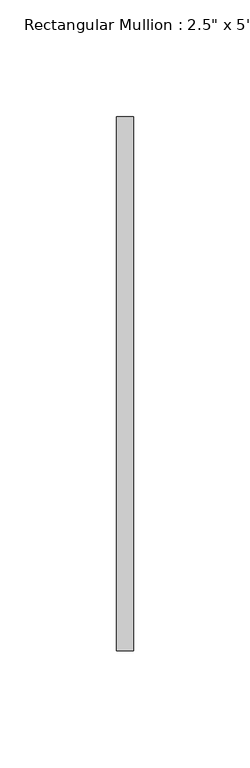
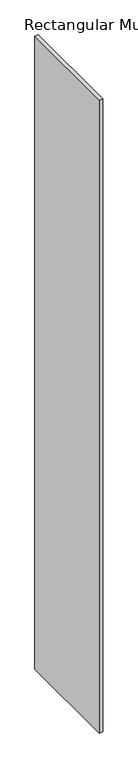
"""IFC4 building model written with IfcOpenShell, lengths in millimetres: member geometry."""

from ifc_helpers import new_model, si_unit, frame, origin, place, context, project, spatial, polyline, outline, extrude, source, transform, mapped, element, save


def member_eaa18777(model_context):
    return source(origin(), model_context, "Body", "SweptSolid", [
        extrude(outline(polyline([(3.6195, 114.3), (3.6195, -114.3), (-3.6195, -114.3), (-3.6195, 114.3), (3.6195, 114.3)])), frame((0.0, 0.0, -1371.6), z_axis=(0.0, 0.0, 1.0), x_axis=(1.0, 0.0, 0.0)), (0.0, 0.0, 1.0), 1371.6),
    ])


if __name__ == "__main__":
    model = new_model("IFC4")
    model_context = context("Model", 3, world=origin())
    ifc_project = project(units=[si_unit("LENGTHUNIT", "METRE", prefix="MILLI")], contexts=[model_context])
    site = spatial("IfcSite", under=ifc_project)
    building = spatial("IfcBuilding", under=site)
    placement = place(None, origin())
    member_shape = member_eaa18777(model_context)
    element("IfcMember", 1, ObjectType="Rectangular Mullion : 2.5\" x 5\" rectangular", at=placement, inside=building, context=model_context, shape_type="MappedRepresentation", body=[
        mapped(member_shape, transform((0.0, 0.0, 0.0), x_axis=(1.0, 0.0, 0.0), y_axis=(0.0, 1.0, 0.0), z_axis=(0.0, 0.0, 1.0))),
    ])
    save(model, "model.ifc")

# Revit data of these elements
# Type "Rectangular Mullion : 2.5\" x 5\" rectangular"
#   built-in parameter 1007304 = 0.75 (stored number, unit not read)
#   built-in parameter 1007301 = 0.011875 (stored number, unit not read)
#   built-in parameter 1007300 = 0.011875 (stored number, unit not read)
# Element 1 (IfcMember, "Rectangular Mullion : 2.5\" x 5\" rectangular")
#   Materials on its faces: "WINDOW GLASS MATERIAL"
# Materials
#   "WINDOW GLASS MATERIAL": class "Generic", colour RGB 120 120 120, transparency 0, Cost = 0
